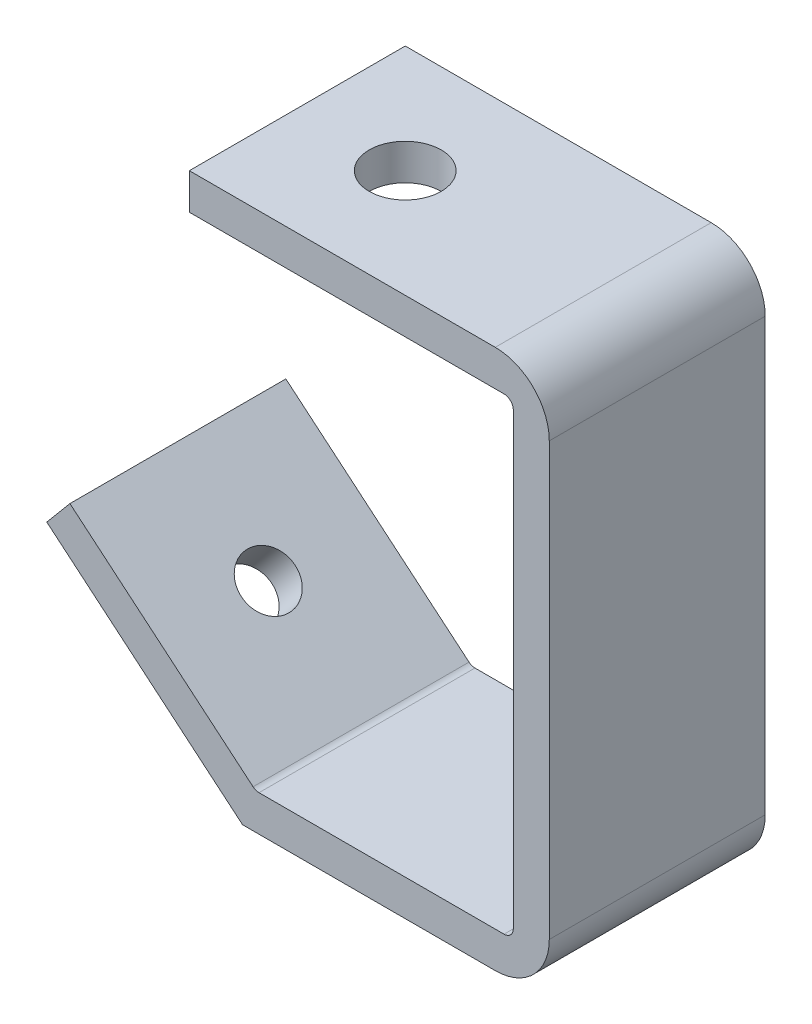
from build123d import *

# Parameters (mm, degrees)
BRACKET_BODY_DEPTH     = 19.05
FLANGE_HOLE_A_SKETCH_R = 6.35
FLANGE_HOLE_A_DEPTH    = 19.05
FLANGE_HOLE_B_SKETCH_R = 4.765
FLANGE_HOLE_B_DEPTH    = 19.05
BEND_FILLET_R1_63_A_R  = 1.63
BEND_FILLET_R1_63_B_R  = 1.63


with BuildPart() as part:
    # Bracket Profile Sketch → Bracket Body (new, symmetric)
    with BuildSketch(Plane.XY):
        with BuildLine():
            Line((0, 0), (44.59, 0))
            ThreePointArc((44.59, 0), (51.328727625, 2.791272375), (54.12, 9.53))
            Line((54.12, 9.53), (54.12, 85.72))
            ThreePointArc((54.12, 85.72), (51.328727625, 92.458727625), (44.59, 95.25))
            Line((44.59, 95.25), (-9.39, 95.25))
            Line((-9.39, 95.25), (-9.39, 88.9))
            Line((-9.39, 88.9), (47.77, 88.9))
            Line((47.77, 88.9), (47.77, 6.35))
            Line((47.77, 6.35), (2.311210988, 6.35))
            Line((2.311210988, 6.35), (-30.459242619, 33.847675535))
            Line((-30.459242619, 33.847675535), (-34.54094394, 28.983293321))
            Line((-34.54094394, 28.983293321), (0, 0))
        make_face()
    extrude(amount=BRACKET_BODY_DEPTH, both=True)

    # Flange Hole A Sketch → Flange Hole A (cut, symmetric)
    with BuildSketch(Plane(origin=(0, 95.25, 0), x_dir=(1, 0, 0), z_dir=(0, 1, 0))):
        with Locations(Location((9.65, 0, 0), (0, 0, 180))):
            Circle(FLANGE_HOLE_A_SKETCH_R)
    extrude(amount=FLANGE_HOLE_A_DEPTH, both=True, mode=Mode.SUBTRACT)

    # Flange Hole B Sketch → Flange Hole B (cut, symmetric)
    with BuildSketch(Plane(origin=(0, 0, 0), x_dir=(0.7660444431189771, -0.6427876096865404, 0), z_dir=(-0.6427876096865404, -0.7660444431189771, 0))):
        with Locations((-24.28, 0)):
            Circle(FLANGE_HOLE_B_SKETCH_R)
    extrude(amount=FLANGE_HOLE_B_DEPTH, both=True, mode=Mode.SUBTRACT)

    # Bend Fillet R1.63 A
    bend_fillet_r1_63_a_edges = [part.edges().sort_by_distance(p)[0] for p in [
        (47.77, 6.35, 0),
        (47.77, 88.9, 0),
    ]]
    fillet(bend_fillet_r1_63_a_edges, radius=BEND_FILLET_R1_63_A_R)

    # Bend Fillet R1.63 B
    bend_fillet_r1_63_b_edges = [part.edges().sort_by_distance(p)[0] for p in [
        (2.311210988, 6.35, 0),
    ]]
    fillet(bend_fillet_r1_63_b_edges, radius=BEND_FILLET_R1_63_B_R)


solid = part.part
